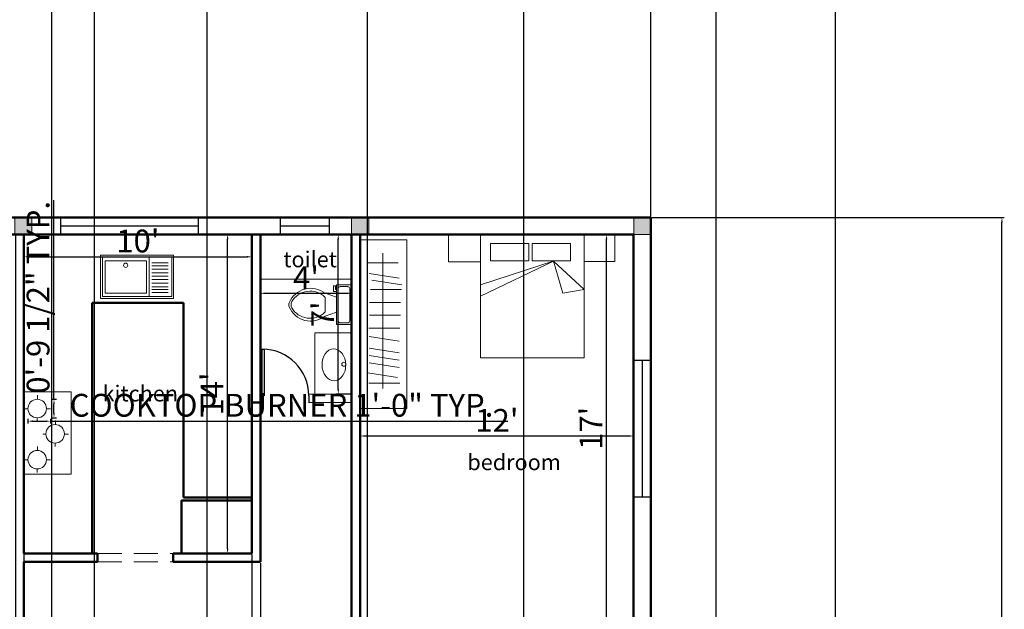
# Model space of a CAD drawing. Units: inches. Extents: x 1367 to 2309, y 1406 to 3826.
# Tile 6 of 9: x 1781 to 2300, y 2608 to 2918. Entities that reach past the tile are written whole.
import ezdxf

# ---------------------------------------------------------------- set-up
doc = ezdxf.new("R2010")
doc.units = ezdxf.units.IN
doc.linetypes.add('DASHED', pattern=[19.05, 12.7, -6.35])
for name, color, linetype, lineweight in [('A-ANNO-DIMS', 2, 'Continuous', 18), ('A-AREA-IDEN', 3, 'Continuous', 18), ('A-DOOR', 4, 'Continuous', 25), ('A-FLOR-FIXT', 8, 'Continuous', 18), ('A-FLOR-OVHD', 8, 'DASHED', 18), ('A-FURN', 8, 'Continuous', 18), ('A-GLAZ', 4, 'Continuous', 25), ('A-WALL', 7, 'Continuous', 50), ('A-WALL-PATT', 8, 'Continuous', 18)]:
    doc.layers.add(name, color=color, linetype=linetype, lineweight=lineweight)
doc.styles.get("Standard").update_dxf_attribs({"font": 'arial.ttf'})
doc.dimstyles.new('ISO-25', dxfattribs={"dimtxt": 12, "dimasz": 2.5, "dimexe": 1.25, "dimexo": 0.625, "dimtad": 1, "dimdec": 0, "dimlunit": 4, "dimtxsty": 'Standard', "dimcen": 2.5, "dimadec": 0, "dimazin": 0, "dimtfac": 1, "dimtdec": 0, "dimtmove": 0, "dimatfit": 3, "dimfxl": 1, "dimarcsym": 0})

# ---------------------------------------------------------------- blocks, each defined once
blk = doc.blocks.new('*U2')
for p, q in [((0, 0), (0, -6)), ((40, 0), (40, -6))]:
    blk.add_line(p, q)
blk.add_lwpolyline([(0, 0), (0, 40), (1.75, 40), (1.75, 0)], close=True)
blk.add_arc((0, 0), 40, 0, 90)
blk = doc.blocks.new('*U4')
for p, q in [((9.5, -6), (9.5, -2)), ((-10, -8.5), (-8, -8.5)), ((-10, -9.5), (-10, -8.5)), ((-7, -9.5), (-10, -9.5)), ((-8, -8.5), (-8, -8)), ((-7, -8), (-7, -9.5)), ((-4, -8), (-6, -14)), ((4, -8), (6, -14)), ((4, -14), (-4, -14))]:
    blk.add_line(p, q)
blk.add_lwpolyline([(10.5, -8), (10.5, 0), (-10.5, 0), (-10.5, -8)], close=True)
for points in [[(-9.5, -2), (-9.5, -6)], [(8.5, -1), (-8.5, -1)], [(-8.5, -7), (8.5, -7)]]:
    blk.add_lwpolyline(points)
for centre, radius, start, end in [((-8.62, -1.88), 0.884, 81.8699, 188.1301), ((8.62, -1.88), 0.884, 351.8699, 98.1301), ((-8.62, -6.12), 0.884, 171.8699, 278.1301), ((8.62, -6.12), 0.884, 261.8699, 8.1301), ((3.52, -21.58), 12.17, 141.4691, 247.9714), ((4.2, -21.82), 11.33, 136.3677, 238.9468), ((-3.52, -21.58), 12.17, 292.0284, 38.5307), ((-4.2, -21.82), 11.33, 301.053, 43.6321), ((0, -27.88), 4, 245.7318, 294.2682), ((0, -29), 4, 254.8605, 285.1395)]:
    blk.add_arc(centre, radius, start, end)
blk = doc.blocks.new('*D11')
at = {"layer": 'A-ANNO-DIMS', "color": 0, "lineweight": -2, "transparency": 16777216}
for p, q in [((1783.37, 2804.54), (1783.37, 2792.2)), ((1903.37, 2804.54), (1903.37, 2792.2)), ((1785.87, 2793.45), (1900.87, 2793.45))]:
    blk.add_line(p, q, dxfattribs=at)
at = {"layer": 'A-ANNO-DIMS', "color": 0, "lineweight": 100, "transparency": 16777216}
for points in [[(1785.87, 2793.87), (1785.87, 2793.04), (1783.37, 2793.45)], [(1900.87, 2793.87), (1900.87, 2793.04), (1903.37, 2793.45)]]:
    blk.add_solid(points, dxfattribs=at)
at = {"layer": 'Defpoints', "color": 0, "lineweight": 100, "transparency": 16777216}
for p in [(1783.37, 2805.17), (1903.37, 2805.17), (1903.37, 2793.45)]:
    blk.add_point(p, dxfattribs=at)
at = {"layer": 'A-ANNO-DIMS', "color": 0, "transparency": 16777216, "insert": (1843.37, 2800.21), "char_height": 12, "attachment_point": 5}
blk.add_mtext("10'", dxfattribs=at)
blk = doc.blocks.new('*D12')
at = {"layer": 'A-ANNO-DIMS', "color": 0, "lineweight": -2, "transparency": 16777216}
for p, q in [((1902.75, 2805.17), (1889.33, 2805.17)), ((1890.58, 2639.81), (1890.58, 2802.67)), ((1902.75, 2637.31), (1889.33, 2637.31))]:
    blk.add_line(p, q, dxfattribs=at)
at = {"layer": 'A-ANNO-DIMS', "color": 0, "lineweight": 100, "transparency": 16777216}
for points in [[(1890.16, 2802.67), (1891, 2802.67), (1890.58, 2805.17)], [(1890.16, 2639.81), (1891, 2639.81), (1890.58, 2637.31)]]:
    blk.add_solid(points, dxfattribs=at)
at = {"layer": 'Defpoints', "color": 0, "lineweight": 100, "transparency": 16777216}
for p in [(1890.58, 2805.17), (1903.37, 2805.17), (1903.37, 2637.31)]:
    blk.add_point(p, dxfattribs=at)
at = {"layer": 'A-ANNO-DIMS', "color": 0, "transparency": 16777216, "insert": (1883.93, 2721.24), "char_height": 12, "attachment_point": 5, "rotation": 90}
blk.add_mtext("14'", dxfattribs=at)
blk = doc.blocks.new('*D13')
at = {"layer": 'A-ANNO-DIMS', "color": 0, "lineweight": -2, "transparency": 16777216}
for p, q in [((1907.87, 2804.54), (1907.87, 2773)), ((1955.87, 2804.54), (1955.87, 2773)), ((1910.37, 2774.25), (1953.37, 2774.25))]:
    blk.add_line(p, q, dxfattribs=at)
at = {"layer": 'A-ANNO-DIMS', "color": 0, "lineweight": 100, "transparency": 16777216}
for points in [[(1910.37, 2774.66), (1910.37, 2773.83), (1907.87, 2774.25)], [(1953.37, 2774.66), (1953.37, 2773.83), (1955.87, 2774.25)]]:
    blk.add_solid(points, dxfattribs=at)
at = {"layer": 'Defpoints', "color": 0, "lineweight": 100, "transparency": 16777216}
for p in [(1907.87, 2805.17), (1955.87, 2805.17), (1955.87, 2774.25)]:
    blk.add_point(p, dxfattribs=at)
at = {"layer": 'A-ANNO-DIMS', "color": 0, "transparency": 16777216, "insert": (1931.87, 2780.87), "char_height": 12, "attachment_point": 5}
blk.add_mtext("4'", dxfattribs=at)
blk = doc.blocks.new('*D14')
at = {"layer": 'A-ANNO-DIMS', "color": 0, "lineweight": -2, "transparency": 16777216}
for p, q in [((1955.25, 2805.17), (1947.61, 2805.17)), ((1948.86, 2723.67), (1948.86, 2802.67)), ((1955.25, 2721.17), (1947.61, 2721.17))]:
    blk.add_line(p, q, dxfattribs=at)
at = {"layer": 'A-ANNO-DIMS', "color": 0, "lineweight": 100, "transparency": 16777216}
for points in [[(1948.45, 2802.67), (1949.28, 2802.67), (1948.86, 2805.17)], [(1948.45, 2723.67), (1949.28, 2723.67), (1948.86, 2721.17)]]:
    blk.add_solid(points, dxfattribs=at)
at = {"layer": 'Defpoints', "color": 0, "lineweight": 100, "transparency": 16777216}
for p in [(1948.86, 2805.17), (1955.87, 2805.17), (1955.87, 2721.17)]:
    blk.add_point(p, dxfattribs=at)
at = {"layer": 'A-ANNO-DIMS', "color": 0, "transparency": 16777216, "insert": (1942.24, 2763.17), "char_height": 12, "attachment_point": 5, "rotation": 90}
blk.add_mtext("7'", dxfattribs=at)
blk = doc.blocks.new('*D15')
at = {"layer": 'A-ANNO-DIMS', "color": 0, "lineweight": -2, "transparency": 16777216}
for p, q in [((1960.37, 2804.54), (1960.37, 2697.87)), ((2104.37, 2804.54), (2104.37, 2697.87)), ((1962.87, 2699.12), (2101.87, 2699.12))]:
    blk.add_line(p, q, dxfattribs=at)
at = {"layer": 'A-ANNO-DIMS', "color": 0, "lineweight": 100, "transparency": 16777216}
for points in [[(1962.87, 2699.54), (1962.87, 2698.71), (1960.37, 2699.12)], [(2101.87, 2699.54), (2101.87, 2698.71), (2104.37, 2699.12)]]:
    blk.add_solid(points, dxfattribs=at)
at = {"layer": 'Defpoints', "color": 0, "lineweight": 100, "transparency": 16777216}
for p in [(1960.37, 2805.17), (2104.37, 2805.17), (2104.37, 2699.12)]:
    blk.add_point(p, dxfattribs=at)
at = {"layer": 'A-ANNO-DIMS', "color": 0, "transparency": 16777216, "insert": (2032.37, 2705.77), "char_height": 12, "attachment_point": 5}
blk.add_mtext("12'", dxfattribs=at)
blk = doc.blocks.new('*D16')
at = {"layer": 'A-ANNO-DIMS', "color": 0, "lineweight": -2, "transparency": 16777216}
for p, q in [((2103.75, 2805.17), (2088.85, 2805.17)), ((2090.1, 2603.67), (2090.1, 2802.67)), ((2103.75, 2601.17), (2088.85, 2601.17))]:
    blk.add_line(p, q, dxfattribs=at)
at = {"layer": 'A-ANNO-DIMS', "color": 0, "lineweight": 100, "transparency": 16777216}
for points in [[(2089.68, 2802.67), (2090.51, 2802.67), (2090.1, 2805.17)], [(2089.68, 2603.67), (2090.51, 2603.67), (2090.1, 2601.17)]]:
    blk.add_solid(points, dxfattribs=at)
at = {"layer": 'Defpoints', "color": 0, "lineweight": 100, "transparency": 16777216}
for p in [(2090.1, 2805.17), (2104.37, 2805.17), (2104.37, 2601.17)]:
    blk.add_point(p, dxfattribs=at)
at = {"layer": 'A-ANNO-DIMS', "color": 0, "transparency": 16777216, "insert": (2083.45, 2703.17), "char_height": 12, "attachment_point": 5, "rotation": 90}
blk.add_mtext("17'", dxfattribs=at)
blk = doc.blocks.new('BURNER')
blk.add_line((9.74, 4.72), (11.92, 4.72))
blk.add_circle((4.87, 4.87), 4.87)
blk = doc.blocks.new('*D47')
at = {"layer": 'A-ANNO-DIMS', "color": 0, "lineweight": -2, "transparency": 16777216}
for p, q in [((1785.48, 2708.07), (1785.48, 2705.66)), ((1787.98, 2706.91), (1794.9, 2706.91)), ((1797.4, 2708.07), (1797.4, 2705.66)), ((1797.4, 2706.91), (2038.09, 2706.91))]:
    blk.add_line(p, q, dxfattribs=at)
at = {"layer": 'A-ANNO-DIMS', "color": 0, "lineweight": 100, "transparency": 16777216}
for points in [[(1787.98, 2707.33), (1787.98, 2706.49), (1785.48, 2706.91)], [(1794.9, 2707.33), (1794.9, 2706.49), (1797.4, 2706.91)]]:
    blk.add_solid(points, dxfattribs=at)
at = {"layer": 'Defpoints', "color": 0, "lineweight": 100, "transparency": 16777216}
for p in [(1785.48, 2708.7), (1797.4, 2708.7), (1797.4, 2706.91)]:
    blk.add_point(p, dxfattribs=at)
at = {"layer": 'A-ANNO-DIMS', "color": 0, "transparency": 16777216, "insert": (1918.99, 2713.74), "char_height": 12, "attachment_point": 5}
blk.add_mtext('COOKTOP BURNER 1\'-0" TYP.', dxfattribs=at)
blk = doc.blocks.new('*D48')
at = {"layer": 'A-ANNO-DIMS', "color": 0, "lineweight": -2, "transparency": 16777216}
for p, q in [((1799.19, 2718.44), (1799.19, 2823.29)), ((1798.02, 2718.44), (1800.44, 2718.44)), ((1799.19, 2711.2), (1799.19, 2715.94)), ((1798.02, 2708.7), (1800.44, 2708.7))]:
    blk.add_line(p, q, dxfattribs=at)
at = {"layer": 'A-ANNO-DIMS', "color": 0, "lineweight": 100, "transparency": 16777216}
for points in [[(1798.77, 2715.94), (1799.6, 2715.94), (1799.19, 2718.44)], [(1798.77, 2711.2), (1799.6, 2711.2), (1799.19, 2708.7)]]:
    blk.add_solid(points, dxfattribs=at)
at = {"layer": 'Defpoints', "color": 0, "lineweight": 100, "transparency": 16777216}
for p in [(1797.4, 2718.44), (1799.19, 2718.44), (1797.4, 2708.7)]:
    blk.add_point(p, dxfattribs=at)
at = {"layer": 'A-ANNO-DIMS', "color": 0, "transparency": 16777216, "insert": (1792.36, 2772.12), "char_height": 12, "attachment_point": 5, "rotation": 90}
blk.add_mtext('0\'-9 1/2" TYP.', dxfattribs=at)
blk = doc.blocks.new('*D87')
at = {"layer": 'A-ANNO-DIMS', "color": 0, "lineweight": -2, "transparency": 16777216}
for p, q in [((1513.37, 2814.79), (1513.37, 3802.6)), ((1515.87, 3801.35), (2110.9, 3801.35)), ((2113.4, 2814.79), (2113.4, 3802.6))]:
    blk.add_line(p, q, dxfattribs=at)
at = {"layer": 'A-ANNO-DIMS', "color": 0, "lineweight": 100, "transparency": 16777216}
for points in [[(1515.87, 3801.77), (1515.87, 3800.93), (1513.37, 3801.35)], [(2110.9, 3801.77), (2110.9, 3800.93), (2113.4, 3801.35)]]:
    blk.add_solid(points, dxfattribs=at)
at = {"layer": 'Defpoints', "color": 0, "lineweight": 100, "transparency": 16777216}
for p in [(2113.4, 3801.35), (1513.37, 2814.17), (2113.4, 2814.17)]:
    blk.add_point(p, dxfattribs=at)
at = {"layer": 'A-ANNO-DIMS', "color": 0, "transparency": 16777216, "insert": (1813.39, 3808.1), "char_height": 12, "attachment_point": 5}
blk.add_mtext('50\'-0"', dxfattribs=at)
blk = doc.blocks.new('*D89')
at = {"layer": 'A-ANNO-DIMS', "color": 0, "lineweight": -2, "transparency": 16777216}
for p, q in [((2114.03, 2814.17), (2299.51, 2814.17)), ((2298.26, 2336.67), (2298.26, 2811.67)), ((2114, 2334.17), (2299.51, 2334.17))]:
    blk.add_line(p, q, dxfattribs=at)
at = {"layer": 'A-ANNO-DIMS', "color": 0, "lineweight": 100, "transparency": 16777216}
for points in [[(2297.84, 2811.67), (2298.67, 2811.67), (2298.26, 2814.17)], [(2297.84, 2336.67), (2298.67, 2336.67), (2298.26, 2334.17)]]:
    blk.add_solid(points, dxfattribs=at)
at = {"layer": 'Defpoints', "color": 0, "lineweight": 100, "transparency": 16777216}
for p in [(2113.4, 2814.17), (2298.26, 2814.17), (2113.37, 2334.17)]:
    blk.add_point(p, dxfattribs=at)
at = {"layer": 'A-ANNO-DIMS', "color": 0, "transparency": 16777216, "insert": (2291.51, 2574.17), "char_height": 12, "attachment_point": 5, "rotation": 90}
blk.add_mtext('40\'-0"', dxfattribs=at)
blk = doc.blocks.new('*D102')
at = {"layer": 'A-ANNO-DIMS', "color": 0, "lineweight": -2, "transparency": 16777216}
for p, q in [((1778.87, 2804.54), (1778.87, 2257.28)), ((1783.37, 2804.54), (1783.37, 2257.28)), ((1776.37, 2258.53), (1773.87, 2258.53)), ((1778.87, 2258.53), (1783.37, 2258.53)), ((1785.87, 2258.53), (1849.48, 2258.53))]:
    blk.add_line(p, q, dxfattribs=at)
at = {"layer": 'A-ANNO-DIMS', "color": 0, "lineweight": 100, "transparency": 16777216}
for points in [[(1776.37, 2258.94), (1776.37, 2258.11), (1778.87, 2258.53)], [(1785.87, 2258.94), (1785.87, 2258.11), (1783.37, 2258.53)]]:
    blk.add_solid(points, dxfattribs=at)
at = {"layer": 'Defpoints', "color": 0, "lineweight": 100, "transparency": 16777216}
for p in [(1778.87, 2805.17), (1783.37, 2805.17), (1783.37, 2258.53)]:
    blk.add_point(p, dxfattribs=at)
at = {"layer": 'A-ANNO-DIMS', "color": 0, "transparency": 16777216, "insert": (1818.93, 2265.35), "char_height": 12, "attachment_point": 5}
blk.add_mtext('0\'-4 1/2"', dxfattribs=at)
blk = doc.blocks.new('*D113')
at = {"layer": 'A-ANNO-DIMS', "color": 0, "lineweight": -2, "transparency": 16777216}
for p, q in [((1797.9, 3128.9), (1797.9, 2257.28)), ((2210.4, 3128.9), (2210.4, 2257.28)), ((1800.4, 2258.53), (2207.9, 2258.53))]:
    blk.add_line(p, q, dxfattribs=at)
at = {"layer": 'A-ANNO-DIMS', "color": 0, "lineweight": 100, "transparency": 16777216}
for points in [[(1800.4, 2258.94), (1800.4, 2258.11), (1797.9, 2258.53)], [(2207.9, 2258.94), (2207.9, 2258.11), (2210.4, 2258.53)]]:
    blk.add_solid(points, dxfattribs=at)
at = {"layer": 'Defpoints', "color": 0, "lineweight": 100, "transparency": 16777216}
for p in [(1797.9, 3129.52), (2210.4, 3129.52), (2210.4, 2258.53)]:
    blk.add_point(p, dxfattribs=at)
at = {"layer": 'A-ANNO-DIMS', "color": 0, "transparency": 16777216, "insert": (2004.15, 2265.36), "char_height": 12, "attachment_point": 5}
blk.add_mtext('34\'-4 1/2"', dxfattribs=at)
blk = doc.blocks.new('*D114')
at = {"layer": 'A-ANNO-DIMS', "color": 0, "lineweight": -2, "transparency": 16777216}
for p, q in [((1820.42, 3150.44), (1820.42, 2257.28)), ((1879.66, 3150.44), (1879.66, 2257.28)), ((1822.92, 2258.53), (1877.16, 2258.53))]:
    blk.add_line(p, q, dxfattribs=at)
at = {"layer": 'A-ANNO-DIMS', "color": 0, "lineweight": 100, "transparency": 16777216}
for points in [[(1822.92, 2258.94), (1822.92, 2258.11), (1820.42, 2258.53)], [(1877.16, 2258.94), (1877.16, 2258.11), (1879.66, 2258.53)]]:
    blk.add_solid(points, dxfattribs=at)
at = {"layer": 'Defpoints', "color": 0, "lineweight": 100, "transparency": 16777216}
for p in [(1820.42, 3151.06), (1879.66, 3151.06), (1879.66, 2258.53)]:
    blk.add_point(p, dxfattribs=at)
at = {"layer": 'A-ANNO-DIMS', "color": 0, "transparency": 16777216, "insert": (1850.04, 2265.17), "char_height": 12, "attachment_point": 5}
blk.add_mtext('4\'-11"', dxfattribs=at)
blk = doc.blocks.new('*D115')
at = {"layer": 'A-ANNO-DIMS', "color": 0, "lineweight": -2, "transparency": 16777216}
for p, q in [((1879.66, 3150.44), (1879.66, 2257.28)), ((1964.13, 3150.44), (1964.13, 2257.28)), ((1882.16, 2258.53), (1961.63, 2258.53))]:
    blk.add_line(p, q, dxfattribs=at)
at = {"layer": 'A-ANNO-DIMS', "color": 0, "lineweight": 100, "transparency": 16777216}
for points in [[(1882.16, 2258.94), (1882.16, 2258.11), (1879.66, 2258.53)], [(1961.63, 2258.94), (1961.63, 2258.11), (1964.13, 2258.53)]]:
    blk.add_solid(points, dxfattribs=at)
at = {"layer": 'Defpoints', "color": 0, "lineweight": 100, "transparency": 16777216}
for p in [(1879.66, 3151.06), (1964.13, 3151.06), (1964.13, 2258.53)]:
    blk.add_point(p, dxfattribs=at)
at = {"layer": 'A-ANNO-DIMS', "color": 0, "transparency": 16777216, "insert": (1921.89, 2265.35), "char_height": 12, "attachment_point": 5}
blk.add_mtext('7\'-0 1/2"', dxfattribs=at)
blk = doc.blocks.new('*D116')
at = {"layer": 'A-ANNO-DIMS', "color": 0, "lineweight": -2, "transparency": 16777216}
for p, q in [((1964.13, 3150.44), (1964.13, 2257.28)), ((2046.46, 3150.44), (2046.46, 2257.28)), ((1966.63, 2258.53), (2043.96, 2258.53))]:
    blk.add_line(p, q, dxfattribs=at)
at = {"layer": 'A-ANNO-DIMS', "color": 0, "lineweight": 100, "transparency": 16777216}
for points in [[(1966.63, 2258.94), (1966.63, 2258.11), (1964.13, 2258.53)], [(2043.96, 2258.94), (2043.96, 2258.11), (2046.46, 2258.53)]]:
    blk.add_solid(points, dxfattribs=at)
at = {"layer": 'Defpoints', "color": 0, "lineweight": 100, "transparency": 16777216}
for p in [(1964.13, 3151.06), (2046.46, 3151.06), (2046.46, 2258.53)]:
    blk.add_point(p, dxfattribs=at)
at = {"layer": 'A-ANNO-DIMS', "color": 0, "transparency": 16777216, "insert": (2005.29, 2265.35), "char_height": 12, "attachment_point": 5}
blk.add_mtext('6\'-10 1/2"', dxfattribs=at)
blk = doc.blocks.new('*D117')
at = {"layer": 'A-ANNO-DIMS', "color": 0, "lineweight": -2, "transparency": 16777216}
for p, q in [((2046.46, 3150.44), (2046.46, 2257.28)), ((2147.64, 3150.44), (2147.64, 2257.28)), ((2048.96, 2258.53), (2145.14, 2258.53))]:
    blk.add_line(p, q, dxfattribs=at)
at = {"layer": 'A-ANNO-DIMS', "color": 0, "lineweight": 100, "transparency": 16777216}
for points in [[(2048.96, 2258.94), (2048.96, 2258.11), (2046.46, 2258.53)], [(2145.14, 2258.94), (2145.14, 2258.11), (2147.64, 2258.53)]]:
    blk.add_solid(points, dxfattribs=at)
at = {"layer": 'Defpoints', "color": 0, "lineweight": 100, "transparency": 16777216}
for p in [(2046.46, 3151.06), (2147.64, 3151.06), (2147.64, 2258.53)]:
    blk.add_point(p, dxfattribs=at)
at = {"layer": 'A-ANNO-DIMS', "color": 0, "transparency": 16777216, "insert": (2097.05, 2265.28), "char_height": 12, "attachment_point": 5}
blk.add_mtext('8\'-5"', dxfattribs=at)
blk = doc.blocks.new('*D135')
at = {"layer": 'A-ANNO-DIMS', "color": 0, "lineweight": -2, "transparency": 16777216}
for p, q in [((1903.37, 2636.69), (1903.37, 2257.28)), ((1907.87, 2632.19), (1907.87, 2257.28)), ((1900.87, 2258.53), (1898.37, 2258.53)), ((1903.37, 2258.53), (1907.87, 2258.53)), ((1910.37, 2258.53), (1973.98, 2258.53))]:
    blk.add_line(p, q, dxfattribs=at)
at = {"layer": 'A-ANNO-DIMS', "color": 0, "lineweight": 100, "transparency": 16777216}
for points in [[(1900.87, 2258.94), (1900.87, 2258.11), (1903.37, 2258.53)], [(1910.37, 2258.94), (1910.37, 2258.11), (1907.87, 2258.53)]]:
    blk.add_solid(points, dxfattribs=at)
at = {"layer": 'Defpoints', "color": 0, "lineweight": 100, "transparency": 16777216}
for p in [(1903.37, 2637.31), (1907.87, 2632.81), (1907.87, 2258.53)]:
    blk.add_point(p, dxfattribs=at)
at = {"layer": 'A-ANNO-DIMS', "color": 0, "transparency": 16777216, "insert": (1943.43, 2265.35), "char_height": 12, "attachment_point": 5}
blk.add_mtext('0\'-4 1/2"', dxfattribs=at)

msp = doc.modelspace()

# ---------------------------------------------------------------- hatches: boundary and pattern name
at = {"layer": 'A-WALL-PATT'}
h = msp.add_hatch(color=256, dxfattribs=at)
h.dxf.hatch_style = 1
h.paths.add_polyline_path([(1513.37, 2983.62), (1504.37, 2983.62), (1504.37, 2974.62), (1513.37, 2974.62)])
h.paths.add_polyline_path([(1759.42, 2983.62), (1749.82, 2983.62), (1749.82, 2974.62), (1759.42, 2974.62)])
h.paths.add_polyline_path([(1513.37, 3283.62), (1504.37, 3283.62), (1504.37, 3274.62), (1513.37, 3274.62)])
h.paths.add_polyline_path([(1759.42, 3283.62), (1750.75, 3283.62), (1750.75, 3274.62), (1759.42, 3274.62)])
h.paths.add_polyline_path([(2113.4, 2983.62), (2104.4, 2983.62), (2104.4, 2974.62), (2113.4, 2974.62)])
h.paths.add_polyline_path([(1787.87, 2343.17), (1778.87, 2343.17), (1778.87, 2334.17), (1787.87, 2334.17)])
h.paths.add_polyline_path([(1964.87, 2343.17), (1960.37, 2343.17), (1955.87, 2343.17), (1955.87, 2334.17), (1964.87, 2334.17)])
h.paths.add_polyline_path([(2113.37, 2343.17), (2104.37, 2343.17), (2104.37, 2334.17), (2113.37, 2334.17)])
h.paths.add_polyline_path([(1783.37, 2513.73), (1774.44, 2513.73), (1774.44, 2504.73), (1783.37, 2504.73)])
h.paths.add_polyline_path([(1787.54, 2814.17), (1778.54, 2814.17), (1778.54, 2805.17), (1787.54, 2805.17)])
h.paths.add_polyline_path([(1964.87, 2814.17), (1955.87, 2814.17), (1955.87, 2805.17), (1964.87, 2805.17)])
h.paths.add_polyline_path([(2113.37, 2814.17), (2104.4, 2814.17), (2104.4, 2805.17), (2113.37, 2805.17)])
h.paths.add_polyline_path([(1522.37, 2814.17), (1513.37, 2814.17), (1513.37, 2805.17), (1522.37, 2805.17)])
h.paths.add_polyline_path([(2019.97, 2440.35), (2070.2, 2440.35), (2070.2, 2457.56), (2019.97, 2457.56)], flags=9)
h.paths.add_polyline_path([(1670.17, 2422.1), (1711.32, 2422.1), (1711.32, 2439.31), (1670.17, 2439.31)], flags=9)
h.paths.add_polyline_path([(1917.64, 2783.38), (1946.46, 2783.38), (1946.46, 2800.59), (1917.64, 2800.59)], flags=9)
h.paths.add_polyline_path([(1526.17, 2423.16), (1570.57, 2423.16), (1570.57, 2440.37), (1526.17, 2440.37)], flags=9)
h.paths.add_polyline_path([(2013.98, 2676.57), (2064.21, 2676.57), (2064.21, 2693.79), (2013.98, 2693.79)], flags=9)
h.paths.add_polyline_path([(1738.47, 2785.04), (1767.29, 2785.04), (1767.29, 2802.25), (1738.47, 2802.25)], flags=9)
h.paths.add_polyline_path([(1832.32, 2473.89), (1889.69, 2473.89), (1889.69, 2491.1), (1832.32, 2491.1)], flags=9)
h.paths.add_polyline_path([(1821.9, 2712.75), (1863.05, 2712.75), (1863.05, 2729.96), (1821.9, 2729.96)], flags=9)
h.paths.add_polyline_path([(1595.64, 2683.62), (1684.77, 2683.62), (1684.77, 2700.83), (1595.64, 2700.83)], flags=9)

# ---------------------------------------------------------------- linework, layer by layer
at = {"layer": 'A-FLOR-OVHD'}
for p, q in [((1822.18, 2637.31), (1861.94, 2637.31)), ((1822.18, 2632.81), (1861.94, 2632.81))]:
    msp.add_line(p, q, dxfattribs=at)
at = {"layer": 'A-FURN'}
for p, q in [((1972.25, 2724.06), (1972.25, 2795.32)), ((1849.37, 2772.51), (1849.37, 2793.34)), ((1850.66, 2790.32), (1859.26, 2790.32)), ((1980.4, 2790.35), (1964.09, 2790.35)), ((2062.49, 2791.33), (2023.67, 2778.61)), ((2062.49, 2791.33), (2023.67, 2772.7)), ((2062.15, 2791.17), (2078.23, 2776.31)), ((2067.01, 2774.36), (2062.15, 2791.17)), ((1850.66, 2788.68), (1859.26, 2788.68)), ((1850.66, 2787), (1859.26, 2787)), ((1850.66, 2785.03), (1859.26, 2785.03)), ((1980.87, 2782.19), (1965.2, 2784.64)), ((1850.66, 2783.17), (1859.26, 2783.17)), ((1850.66, 2781.43), (1859.26, 2781.43)), ((1850.66, 2779.58), (1859.26, 2779.58)), ((1955.87, 2781.67), (1907.87, 2781.67)), ((1982.28, 2778.72), (1966.61, 2781.18)), ((1850.66, 2777.72), (1859.26, 2777.72)), ((1850.66, 2776.26), (1859.26, 2776.26)), ((1850.66, 2774.58), (1859.26, 2774.58)), ((1982.15, 2776.27), (1965.83, 2776.27)), ((2078.23, 2776.31), (2067.01, 2774.36)), ((1981.68, 2769.35), (1965.37, 2769.35)), ((1981.68, 2762.66), (1965.37, 2762.66)), ((1981.18, 2755.96), (1964.86, 2755.96)), ((1980.87, 2749.07), (1965.2, 2751.53)), ((1980.87, 2742.94), (1965.2, 2745.4)), ((1980.87, 2739.06), (1965.2, 2741.52)), ((1980.87, 2735.18), (1965.2, 2737.64)), ((1980.02, 2729.86), (1964.36, 2732.31)), ((1981.18, 2726.97), (1964.86, 2726.97)), ((1967.61, 2726.97), (1981.18, 2726.97)), ((1790.58, 2718.43), (1790.58, 2720.57)), ((1955.87, 2721.17), (1933.17, 2721.17)), ((1955.87, 2716.67), (1933.18, 2716.67)), ((1933.31, 2721.17), (1955.87, 2721.17)), ((1933.33, 2716.67), (1955.87, 2716.67)), ((1785.48, 2713.42), (1783.91, 2713.42)), ((1790.41, 2708.7), (1790.41, 2706.83)), ((1800.02, 2705.11), (1800.02, 2707.25)), ((1794.93, 2700.1), (1793.35, 2700.1)), ((1790.58, 2691.51), (1790.58, 2693.66)), ((1799.85, 2695.38), (1799.85, 2693.51)), ((1785.48, 2686.5), (1783.91, 2686.5)), ((1790.41, 2681.78), (1790.41, 2679.91))]:
    msp.add_line(p, q, dxfattribs=at)
for points in [[(1778.54, 2814.17), (1787.54, 2814.17), (1787.54, 2805.17), (1778.54, 2805.17)], [(1955.87, 2814.17), (1964.87, 2814.17), (1964.87, 2805.17), (1955.87, 2805.17)], [(2104.4, 2814.17), (2113.4, 2814.17), (2113.4, 2805.17), (2104.4, 2805.17)], [(2023.67, 2805.17), (2006.85, 2805.17), (2006.85, 2790.76), (2023.67, 2790.76)], [(2023.67, 2805.17), (2078.23, 2805.17), (2078.23, 2740.23), (2023.67, 2740.23)], [(2078.23, 2805.17), (2094.5, 2805.17), (2094.5, 2790.9), (2078.23, 2790.9)], [(1960.37, 2713.51), (1985.01, 2713.51), (1985.01, 2802.36), (1960.37, 2802.36)], [(2029.04, 2800.54), (2049.23, 2800.54), (2049.23, 2791.33), (2029.04, 2791.33)], [(2050.91, 2800.54), (2071.1, 2800.54), (2071.1, 2791.33), (2050.91, 2791.33)], [(1823.65, 2771.51), (1862.16, 2771.51), (1862.16, 2794.34), (1823.65, 2794.34)], [(1824.65, 2772.51), (1861.16, 2772.51), (1861.16, 2793.34), (1824.65, 2793.34)], [(1826.08, 2791.27), (1847.85, 2791.27), (1847.85, 2774.35), (1826.08, 2774.35)], [(1936.52, 2721.17), (1955.87, 2721.17), (1955.87, 2753.34), (1936.52, 2753.34)], [(1783.37, 2679), (1808.19, 2679), (1808.19, 2722.38), (1783.37, 2722.38)]]:
    msp.add_lwpolyline(points, close=True, dxfattribs=at)
for centre, radius in [((1836.93, 2789.02), 1.12), ((1951.77, 2736.86), 1.06)]:
    msp.add_circle(centre, radius, dxfattribs=at)
msp.add_ellipse((1946.56, 2736.6), major_axis=(-0.17, 8.38), ratio=0.747916, dxfattribs=at)
at = {"layer": 'A-GLAZ'}
for p, q in [((1802.87, 2809.67), (1875.03, 2809.67)), ((1918.21, 2809.67), (1944.28, 2809.67)), ((2108.87, 2739.12), (2108.87, 2666.96))]:
    msp.add_line(p, q, dxfattribs=at)
for points in [[(1802.87, 2814.17), (1875.03, 2814.17), (1875.03, 2805.17), (1802.87, 2805.17)], [(1918.21, 2805.17), (1944.28, 2805.17), (1944.28, 2814.17), (1918.21, 2814.17)], [(2113.37, 2739.12), (2113.37, 2666.96), (2104.37, 2666.96), (2104.37, 2739.12)]]:
    msp.add_lwpolyline(points, close=True, dxfattribs=at)
at = {"layer": 'A-WALL'}
for p, q in [((1783.37, 2637.31), (1783.37, 2805.17)), ((1901.26, 2805.17), (1853.26, 2805.17)), ((2090.75, 2805.17), (1901.26, 2805.17)), ((1903.37, 2805.17), (1903.37, 2716.67)), ((1903.37, 2805.17), (1903.37, 2637.31)), ((1903.37, 2805.17), (1903.37, 2769.17)), ((1955.87, 2805.17), (1907.87, 2805.17)), ((1907.87, 2805.17), (1907.87, 2721.17)), ((1907.87, 2805.17), (1907.87, 2632.81)), ((1955.87, 2805.17), (1955.87, 2596.67)), ((1960.37, 2805.17), (1960.37, 2601.17)), ((2104.37, 2805.17), (1984.37, 2805.17)), ((1819.37, 2637.31), (1819.37, 2769.17)), ((1867.37, 2769.17), (1819.37, 2769.17)), ((1867.37, 2666.69), (1867.37, 2769.17)), ((1903.37, 2716.67), (1908.84, 2716.67)), ((1907.87, 2721.17), (1909.91, 2721.17)), ((1903.37, 2666.69), (1867.37, 2666.69)), ((1783.37, 2637.31), (1807.37, 2637.31)), ((1822.18, 2637.31), (1783.37, 2637.31)), ((1807.37, 2637.31), (1819.37, 2637.31)), ((1822.18, 2637.31), (1822.18, 2632.81)), ((1903.37, 2637.31), (1861.94, 2637.31)), ((1861.94, 2637.31), (1861.94, 2632.81)), ((1783.37, 2601.17), (1783.37, 2632.81)), ((1822.18, 2632.81), (1783.37, 2632.81)), ((1907.87, 2632.81), (1861.94, 2632.81))]:
    msp.add_line(p, q, dxfattribs=at)
for points in [[(1513.37, 2334.17), (2113.37, 2334.17), (2113.37, 2814.17), (1513.37, 2814.17)], [(1903.37, 2637.31), (1866.37, 2637.31), (1866.37, 2665.12), (1903.37, 2665.12)]]:
    msp.add_lwpolyline(points, close=True, dxfattribs=at)
msp.add_lwpolyline([(2104.37, 2511.66), (2104.37, 2805.17), (1522.37, 2805.17), (1522.37, 2507.16)], dxfattribs=at)

# ---------------------------------------------------------------- block references
at = {"layer": 'A-DOOR', "xscale": 0.6122238826041507, "yscale": 0.6122238826041507, "zscale": 0.6122238826041507}
msp.add_blockref('*U2', (1908.84, 2720.34), dxfattribs=at)
at = {"layer": 'A-FLOR-FIXT', "rotation": 270}
msp.add_blockref('*U4', (1955.87, 2768.23), dxfattribs=at)
at = {"layer": 'A-FLOR-FIXT'}
for p in [(1785.48, 2708.7), (1794.92, 2695.38), (1785.48, 2681.78)]:
    msp.add_blockref('BURNER', p, dxfattribs=at)

# ---------------------------------------------------------------- texts
at = {"layer": 'A-AREA-IDEN', "char_height": 8.353, "attachment_point": 1}
for s, insert in [('toilet', (1919.93, 2796.29)), ('kitchen', (1824.76, 2725.66)), ('bedroom', (2016.83, 2689.49))]:
    msp.add_mtext_dynamic_manual_height_columns(s, width=204.251, gutter_width=41.76, heights=[0], dxfattribs=dict(at, insert=insert))

# ---------------------------------------------------------------- dimensions: what is measured, and where the dimension line sits
at = {"layer": 'A-ANNO-DIMS'}
for base, p1, p2, override, picture, middle in [((2113.4, 3801.35), (1513.37, 2814.17), (2113.4, 2814.17), {"dimdec": 1, "dimlfac": 1, "dimrnd": 0, "dimzin": 1, "dimdsep": 46, "dimlunit": 4, "dimfrac": 2}, '*D87', (1813.39, 3808.1)), ((1879.66, 2258.53), (1820.42, 3151.06), (1879.66, 3151.06), {"dimdec": 1, "dimlfac": 1, "dimrnd": 0, "dimzin": 1, "dimdsep": 46, "dimlunit": 4, "dimfrac": 2}, '*D114', (1850.04, 2265.17)), ((1964.13, 2258.53), (1879.66, 3151.06), (1964.13, 3151.06), {"dimdec": 1, "dimlfac": 1, "dimrnd": 0, "dimzin": 1, "dimdsep": 46, "dimlunit": 4, "dimfrac": 2}, '*D115', (1921.89, 2265.35)), ((2046.46, 2258.53), (1964.13, 3151.06), (2046.46, 3151.06), {"dimdec": 1, "dimlfac": 1, "dimrnd": 0, "dimzin": 1, "dimdsep": 46, "dimlunit": 4, "dimfrac": 2}, '*D116', (2005.29, 2265.35)), ((2147.64, 2258.53), (2046.46, 3151.06), (2147.64, 3151.06), {"dimdec": 1, "dimlfac": 1, "dimrnd": 0, "dimzin": 1, "dimdsep": 46, "dimlunit": 4, "dimfrac": 2}, '*D117', (2097.05, 2265.28)), ((2210.4, 2258.53), (1797.9, 3129.52), (2210.4, 3129.52), {"dimdec": 1, "dimlfac": 1, "dimrnd": 0, "dimzin": 1, "dimdsep": 46, "dimlunit": 4, "dimfrac": 2}, '*D113', (2004.15, 2265.36)), ((1783.37, 2258.53), (1778.87, 2805.17), (1783.37, 2805.17), {"dimdec": 1, "dimlfac": 1, "dimrnd": 0, "dimzin": 1, "dimdsep": 46, "dimlunit": 4, "dimfrac": 2}, '*D102', (1818.93, 2265.35)), ((1903.37, 2793.45), (1783.37, 2805.17), (1903.37, 2805.17), {"dimclrd": 0, "dimclre": 0, "dimclrt": 0}, '*D11', (1843.37, 2800.21)), ((1955.87, 2774.25), (1907.87, 2805.17), (1955.87, 2805.17), {"dimclrd": 0, "dimclre": 0, "dimclrt": 0}, '*D13', (1931.87, 2780.87)), ((2104.37, 2699.12), (1960.37, 2805.17), (2104.37, 2805.17), {"dimclrd": 0, "dimclre": 0, "dimclrt": 0}, '*D15', (2032.37, 2705.77)), ((1907.87, 2258.53), (1903.37, 2637.31), (1907.87, 2632.81), {"dimdec": 1, "dimlfac": 1, "dimrnd": 0, "dimzin": 1, "dimdsep": 46, "dimlunit": 4, "dimfrac": 2}, '*D135', (1943.43, 2265.35))]:
    dim = msp.add_linear_dim(base=base, p1=p1, p2=p2, dimstyle='ISO-25', override=override, dxfattribs=at)
    dim.commit()
    dim.dimension.update_dxf_attribs({"geometry": picture, "text_midpoint": middle})
dim = msp.add_linear_dim(base=(1799.19, 2718.44), p1=(1797.4, 2708.7), p2=(1797.4, 2718.44), angle=90, text='<> TYP.', dimstyle='ISO-25', override={"dimdec": 1, "dimrnd": 0, "dimzin": 1, "dimlunit": 4, "dimfrac": 2}, dxfattribs=at)
dim.commit()
dim.dimension.update_dxf_attribs({"geometry": '*D48', "text_midpoint": (1792.36, 2772.12)})
for base, p1, p2, override, picture, middle in [((2298.26, 2814.17), (2113.37, 2334.17), (2113.4, 2814.17), {"dimdec": 1, "dimlfac": 1, "dimrnd": 0, "dimzin": 1, "dimdsep": 46, "dimlunit": 4, "dimfrac": 2}, '*D89', (2291.51, 2574.17)), ((1890.58, 2805.17), (1903.37, 2637.31), (1903.37, 2805.17), {"dimclrd": 0, "dimclre": 0, "dimclrt": 0}, '*D12', (1883.93, 2721.24)), ((1948.86, 2805.17), (1955.87, 2721.17), (1955.87, 2805.17), {"dimclrd": 0, "dimclre": 0, "dimclrt": 0}, '*D14', (1942.24, 2763.17)), ((2090.1, 2805.17), (2104.37, 2601.17), (2104.37, 2805.17), {"dimclrd": 0, "dimclre": 0, "dimclrt": 0}, '*D16', (2083.45, 2703.17))]:
    dim = msp.add_linear_dim(base=base, p1=p1, p2=p2, angle=90, dimstyle='ISO-25', override=override, dxfattribs=at)
    dim.commit()
    dim.dimension.update_dxf_attribs({"geometry": picture, "text_midpoint": middle})
dim = msp.add_linear_dim(base=(1797.4, 2706.91), p1=(1785.48, 2708.7), p2=(1797.4, 2708.7), text='COOKTOP BURNER <> TYP.', dimstyle='ISO-25', override={"dimdec": 1, "dimrnd": 0, "dimzin": 1, "dimlunit": 4, "dimfrac": 2}, dxfattribs=at)
dim.commit()
dim.dimension.update_dxf_attribs({"geometry": '*D47', "text_midpoint": (1918.99, 2713.74)})

doc.saveas('drawing.dxf')
